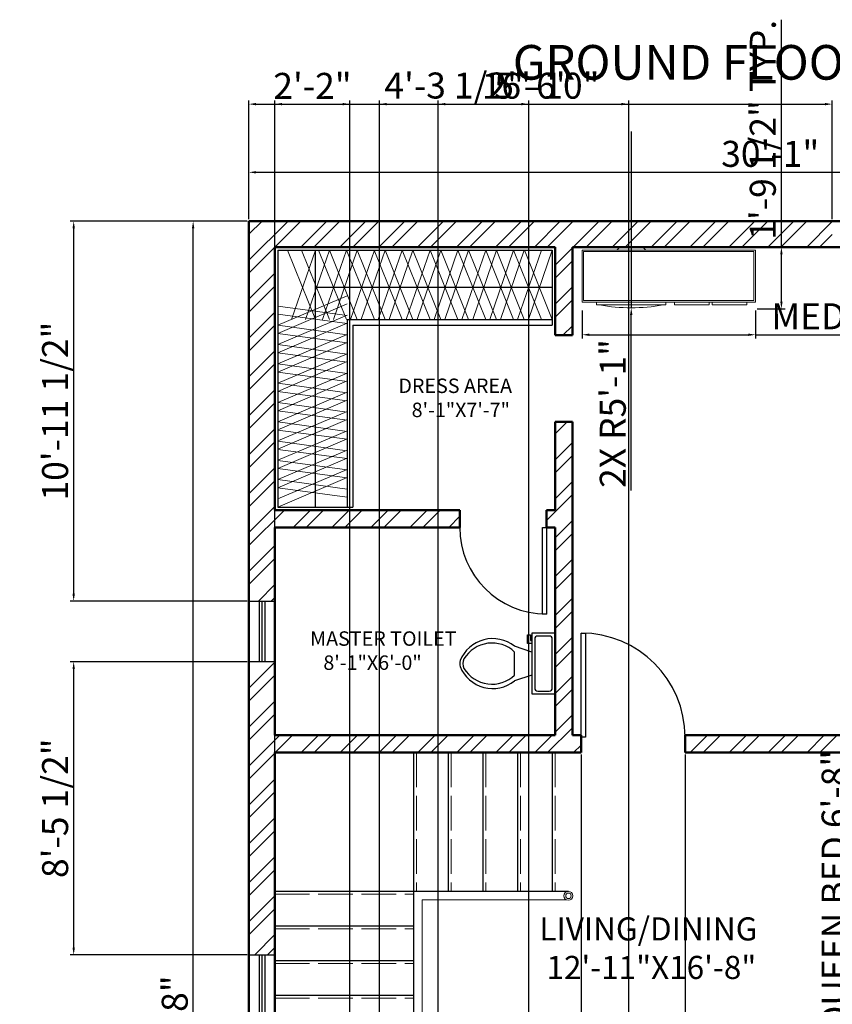
# Model space of a CAD drawing. Units: inches. Extents: x 635 to 1184, y 1837 to 2697.
# Tile 5 of 6: x 635 to 916, y 2356 to 2697. Entities that reach past the tile are written whole.
import ezdxf

# ---------------------------------------------------------------- set-up
doc = ezdxf.new("R2010")
doc.units = ezdxf.units.IN
doc.linetypes.add('ACAD_ISO02W100', pattern=[15, 12, -3])
for name, color, linetype, lineweight in [('A-ANNO-DIMS', 2, 'Continuous', 18), ('A-ANNO-TEXT', 7, 'Continuous', 25), ('A-AREA-IDEN', 7, 'Continuous', 25), ('A-CSWK', 8, 'Continuous', 25), ('A-CSWK-PATT', 252, 'Continuous', 13), ('A-DOOR', 4, 'Continuous', 25), ('A-FLOR-FIXT', 8, 'Continuous', 25), ('A-FLOR-RAIL', 7, 'Continuous', 18), ('A-FLOR-STRS', 7, 'Continuous', 25), ('A-FLOR-STRS-HIDN', 8, 'ACAD_ISO02W100', 13), ('A-FURN', 8, 'Continuous', 18), ('A-GLAZ', 244, 'Continuous', 25), ('A-WALL', 7, 'Continuous', 50), ('A-WALL-PATT', 252, 'Continuous', 13)]:
    doc.layers.add(name, color=color, linetype=linetype, lineweight=lineweight)
doc.styles.get("Standard").update_dxf_attribs({"font": 'arial.ttf'})
doc.dimstyles.new('ISO-25', dxfattribs={"dimtxt": 9, "dimasz": 2.5, "dimexe": 1.25, "dimexo": 0.625, "dimtad": 1, "dimlunit": 3, "dimtxsty": 'Standard', "dimcen": 2.5, "dimadec": 0, "dimazin": 0, "dimtfac": 1, "dimtmove": 0, "dimatfit": 3, "dimfxl": 1, "dimarcsym": 0})

# ---------------------------------------------------------------- blocks, each defined once
blk = doc.blocks.new('*U3')
for p, q in [((0, 0), (0, -6)), ((40, 0), (40, -6))]:
    blk.add_line(p, q)
blk.add_lwpolyline([(0, 0), (0, 40), (1.75, 40), (1.75, 0)], close=True)
blk.add_arc((0, 0), 40, 0, 90)
blk = doc.blocks.new('*U5')
for p, q in [((-40, 0), (-40, 6)), ((0, 0), (0, 6))]:
    blk.add_line(p, q)
blk.add_lwpolyline([(0, 0), (0, -40), (-1.75, -40), (-1.75, 0)], close=True)
blk.add_arc((0, 0), 40, 180, 270)
blk = doc.blocks.new('*U8')
for p, q in [((9.5, -6), (9.5, -2)), ((-10, -8.5), (-8, -8.5)), ((-10, -9.5), (-10, -8.5)), ((-7, -9.5), (-10, -9.5)), ((-8, -8.5), (-8, -8)), ((-7, -8), (-7, -9.5)), ((-4, -8), (-6, -14)), ((4, -8), (6, -14)), ((4, -14), (-4, -14))]:
    blk.add_line(p, q)
blk.add_lwpolyline([(10.5, -8), (10.5, 0), (-10.5, 0), (-10.5, -8)], close=True)
for points in [[(-9.5, -2), (-9.5, -6)], [(8.5, -1), (-8.5, -1)], [(-8.5, -7), (8.5, -7)]]:
    blk.add_lwpolyline(points)
for centre, radius, start, end in [((-8.62, -1.88), 0.884, 81.8699, 188.1301), ((8.62, -1.88), 0.884, 351.8699, 98.1301), ((-8.62, -6.12), 0.884, 171.8699, 278.1301), ((8.62, -6.12), 0.884, 261.8699, 8.1301), ((3.52, -21.58), 12.17, 141.4691, 247.9714), ((4.2, -21.82), 11.33, 136.3677, 238.9468), ((-3.52, -21.58), 12.17, 292.0284, 38.5307), ((-4.2, -21.82), 11.33, 301.053, 43.6321), ((0, -27.88), 4, 245.7318, 294.2682), ((0, -29), 4, 254.8605, 285.1395)]:
    blk.add_arc(centre, radius, start, end)
blk = doc.blocks.new('Entertainment Center')
for p, q in [((-4, 0), (-5, -1)), ((4, 0), (-4, 0)), ((5, -1), (4, 0)), ((-17, -19), (-17, -1)), ((-17, -1), (43, -1)), ((-16.5, -18.5), (-16.5, -1.5)), ((-16.5, -1.5), (42.5, -1.5)), ((42.5, -1.5), (42.5, -18.5)), ((43, -1), (43, -19)), ((43, -19), (-17, -19)), ((42.5, -18.5), (-16.5, -18.5)), ((-12, -20), (-12, -19)), ((12, -20), (-12, -20)), ((12, -19), (12, -20)), ((15, -20), (15, -19)), ((27, -20), (15, -20)), ((27, -19), (27, -20)), ((28, -20), (28, -19)), ((40, -20), (28, -20)), ((40, -19), (40, -20))]:
    blk.add_line(p, q)
blk.add_arc((0, 40), 61, 259.6111, 280.3889)
blk = doc.blocks.new('*D17')
at = {"layer": 'A-ANNO-DIMS', "color": 0, "lineweight": -2, "transparency": 16777216}
for p, q in [((713.66, 2627.14), (693.72, 2627.14)), ((694.97, 2056.46), (694.97, 2624.64)), ((713.66, 2053.96), (693.72, 2053.96))]:
    blk.add_line(p, q, dxfattribs=at)
at = {"layer": 'A-ANNO-DIMS', "color": 0, "transparency": 16777216}
for points in [[(694.56, 2624.64), (695.39, 2624.64), (694.97, 2627.14)], [(694.56, 2056.46), (695.39, 2056.46), (694.97, 2053.96)]]:
    blk.add_solid(points, dxfattribs=at)
at = {"layer": 'DEFPOINTS', "color": 0, "transparency": 16777216}
for p in [(694.97, 2627.14), (714.28, 2627.14), (714.28, 2053.96)]:
    blk.add_point(p, dxfattribs=at)
at = {"layer": 'A-ANNO-DIMS', "color": 0, "transparency": 16777216, "insert": (689.75, 2340.55), "char_height": 9, "attachment_point": 5, "rotation": 90}
blk.add_mtext('47\'-9.18"', dxfattribs=at)
blk = doc.blocks.new('*D18')
at = {"layer": 'A-ANNO-DIMS', "color": 0, "lineweight": -2, "transparency": 16777216}
for p, q in [((714.28, 2627.77), (714.28, 2645.3)), ((1075.28, 2627.77), (1075.28, 2645.3)), ((716.78, 2644.05), (1072.78, 2644.05))]:
    blk.add_line(p, q, dxfattribs=at)
at = {"layer": 'A-ANNO-DIMS', "color": 0, "transparency": 16777216}
for points in [[(716.78, 2644.46), (716.78, 2643.63), (714.28, 2644.05)], [(1072.78, 2644.46), (1072.78, 2643.63), (1075.28, 2644.05)]]:
    blk.add_solid(points, dxfattribs=at)
at = {"layer": 'DEFPOINTS', "color": 0, "transparency": 16777216}
for p in [(1075.28, 2644.05), (714.28, 2627.14), (1075.28, 2627.14)]:
    blk.add_point(p, dxfattribs=at)
at = {"layer": 'A-ANNO-DIMS', "color": 0, "transparency": 16777216, "insert": (894.78, 2649.27), "char_height": 9, "attachment_point": 5}
blk.add_mtext('30\'-1"', dxfattribs=at)
blk = doc.blocks.new('WIN-21IN')
for p, q in [((3.5, 21), (3.5, 0)), ((4.5, 21), (4.5, 0)), ((5.5, 21), (5.5, 0))]:
    blk.add_line(p, q)
blk.add_lwpolyline([(0, 21), (9, 21), (9, 0), (0, 0)], close=True)
blk = doc.blocks.new('WIN-60IN')
for p, q in [((0, 5.5), (60, 5.5)), ((0, 4.5), (60, 4.5)), ((0, 3.5), (60, 3.5))]:
    blk.add_line(p, q)
blk.add_lwpolyline([(0, 9), (60, 9), (60, 0), (0, 0)], close=True)
blk = doc.blocks.new('*D29')
at = {"layer": 'A-ANNO-DIMS', "color": 0, "lineweight": -2, "transparency": 16777216}
for p, q in [((829.66, 2596.18), (829.66, 2586.56)), ((889.66, 2596.18), (889.66, 2586.56)), ((832.16, 2587.81), (887.16, 2587.81)), ((889.66, 2587.81), (1024, 2587.81))]:
    blk.add_line(p, q, dxfattribs=at)
at = {"layer": 'A-ANNO-DIMS', "color": 0, "transparency": 16777216}
for points in [[(832.16, 2588.23), (832.16, 2587.39), (829.66, 2587.81)], [(887.16, 2588.23), (887.16, 2587.39), (889.66, 2587.81)]]:
    blk.add_solid(points, dxfattribs=at)
at = {"layer": 'DEFPOINTS', "color": 0, "transparency": 16777216}
for p in [(829.66, 2596.81), (889.66, 2596.81), (889.66, 2587.81)]:
    blk.add_point(p, dxfattribs=at)
at = {"layer": 'A-ANNO-DIMS', "color": 0, "transparency": 16777216, "insert": (958.08, 2593.03), "char_height": 9, "attachment_point": 5}
blk.add_mtext('MEDIA UNIT 5\'-0" TYP.', dxfattribs=at)
blk = doc.blocks.new('*D30')
at = {"layer": 'A-ANNO-DIMS', "color": 0, "lineweight": -2, "transparency": 16777216}
for p, q in [((898.66, 2618.14), (898.66, 2696.88)), ((890.29, 2618.14), (899.91, 2618.14)), ((898.66, 2599.31), (898.66, 2615.64)), ((890.29, 2596.81), (899.91, 2596.81))]:
    blk.add_line(p, q, dxfattribs=at)
at = {"layer": 'A-ANNO-DIMS', "color": 0, "transparency": 16777216}
for points in [[(898.25, 2615.64), (899.08, 2615.64), (898.66, 2618.14)], [(898.25, 2599.31), (899.08, 2599.31), (898.66, 2596.81)]]:
    blk.add_solid(points, dxfattribs=at)
at = {"layer": 'DEFPOINTS', "color": 0, "transparency": 16777216}
for p in [(889.66, 2618.14), (898.66, 2618.14), (889.66, 2596.81)]:
    blk.add_point(p, dxfattribs=at)
at = {"layer": 'A-ANNO-DIMS', "color": 0, "transparency": 16777216, "insert": (893.38, 2658.76), "char_height": 9, "attachment_point": 5, "rotation": 90}
blk.add_mtext('1\'-9 1/2" TYP.', dxfattribs=at)
blk = doc.blocks.new('*D35')
at = {"layer": 'A-ANNO-DIMS', "color": 0, "lineweight": -2, "transparency": 16777216}
for p, q in [((935.16, 2529.14), (922.53, 2529.14)), ((923.78, 2526.64), (923.78, 2451.64)), ((935.16, 2449.14), (922.53, 2449.14)), ((923.78, 2449.14), (923.78, 2343.94))]:
    blk.add_line(p, q, dxfattribs=at)
at = {"layer": 'A-ANNO-DIMS', "color": 0, "transparency": 16777216}
for points in [[(923.37, 2526.64), (924.2, 2526.64), (923.78, 2529.14)], [(923.37, 2451.64), (924.2, 2451.64), (923.78, 2449.14)]]:
    blk.add_solid(points, dxfattribs=at)
at = {"layer": 'DEFPOINTS', "color": 0, "transparency": 16777216}
for p in [(935.78, 2529.14), (923.78, 2449.14), (935.78, 2449.14)]:
    blk.add_point(p, dxfattribs=at)
at = {"layer": 'A-ANNO-DIMS', "color": 0, "transparency": 16777216, "insert": (918.23, 2395.29), "char_height": 9, "attachment_point": 5, "rotation": 90}
blk.add_mtext('QUEEN BED 6\'-8"', dxfattribs=at)
blk = doc.blocks.new('*D42')
at = {"layer": 'A-ANNO-DIMS', "color": 0, "lineweight": -2, "transparency": 16777216}
for p, q in [((713.66, 2474.64), (652.36, 2474.64)), ((653.61, 2375.64), (653.61, 2472.14)), ((713.66, 2373.14), (652.36, 2373.14))]:
    blk.add_line(p, q, dxfattribs=at)
at = {"layer": 'A-ANNO-DIMS', "color": 0, "transparency": 16777216}
for points in [[(653.2, 2472.14), (654.03, 2472.14), (653.61, 2474.64)], [(653.2, 2375.64), (654.03, 2375.64), (653.61, 2373.14)]]:
    blk.add_solid(points, dxfattribs=at)
at = {"layer": 'DEFPOINTS', "color": 0, "transparency": 16777216}
for p in [(653.61, 2474.64), (714.28, 2474.64), (714.28, 2373.14)]:
    blk.add_point(p, dxfattribs=at)
at = {"layer": 'A-ANNO-DIMS', "color": 0, "transparency": 16777216, "insert": (648.34, 2423.89), "char_height": 9, "attachment_point": 5, "rotation": 90}
blk.add_mtext('8\'-5 1/2"', dxfattribs=at)
blk = doc.blocks.new('*D43')
at = {"layer": 'A-ANNO-DIMS', "color": 0, "lineweight": -2, "transparency": 16777216}
for p, q in [((713.66, 2627.14), (652.36, 2627.14)), ((653.61, 2498.14), (653.61, 2624.64)), ((713.66, 2495.64), (652.36, 2495.64))]:
    blk.add_line(p, q, dxfattribs=at)
at = {"layer": 'A-ANNO-DIMS', "color": 0, "transparency": 16777216}
for points in [[(653.2, 2624.64), (654.03, 2624.64), (653.61, 2627.14)], [(653.2, 2498.14), (654.03, 2498.14), (653.61, 2495.64)]]:
    blk.add_solid(points, dxfattribs=at)
at = {"layer": 'DEFPOINTS', "color": 0, "transparency": 16777216}
for p in [(653.61, 2627.14), (714.28, 2627.14), (714.28, 2495.64)]:
    blk.add_point(p, dxfattribs=at)
at = {"layer": 'A-ANNO-DIMS', "color": 0, "transparency": 16777216, "insert": (648.34, 2561.39), "char_height": 9, "attachment_point": 5, "rotation": 90}
blk.add_mtext('10\'-11 1/2"', dxfattribs=at)
blk = doc.blocks.new('*D44')
at = {"layer": 'A-ANNO-DIMS', "color": 0, "lineweight": -2, "transparency": 16777216}
for p, q in [((714.28, 2627.77), (714.28, 2668.89)), ((916.28, 2627.77), (916.28, 2668.89)), ((716.78, 2667.64), (913.78, 2667.64))]:
    blk.add_line(p, q, dxfattribs=at)
at = {"layer": 'A-ANNO-DIMS', "color": 0, "transparency": 16777216}
for points in [[(716.78, 2668.06), (716.78, 2667.23), (714.28, 2667.64)], [(913.78, 2668.06), (913.78, 2667.23), (916.28, 2667.64)]]:
    blk.add_solid(points, dxfattribs=at)
at = {"layer": 'DEFPOINTS', "color": 0, "transparency": 16777216}
for p in [(916.28, 2667.64), (714.28, 2627.14), (916.28, 2627.14)]:
    blk.add_point(p, dxfattribs=at)
at = {"layer": 'A-ANNO-DIMS', "color": 0, "transparency": 16777216, "insert": (815.28, 2672.86), "char_height": 9, "attachment_point": 5}
blk.add_mtext('16\'-10"', dxfattribs=at)
blk = doc.blocks.new('*D56')
at = {"layer": 'A-ANNO-DIMS', "color": 0, "lineweight": -2, "transparency": 16777216}
for p, q in [((759.51, 2116.34), (759.51, 2668.89)), ((811.15, 2116.34), (811.15, 2668.89)), ((762.01, 2667.64), (808.65, 2667.64))]:
    blk.add_line(p, q, dxfattribs=at)
at = {"layer": 'A-ANNO-DIMS', "color": 0, "transparency": 16777216}
for points in [[(762.01, 2668.06), (762.01, 2667.23), (759.51, 2667.64)], [(808.65, 2668.06), (808.65, 2667.23), (811.15, 2667.64)]]:
    blk.add_solid(points, dxfattribs=at)
at = {"layer": 'DEFPOINTS', "color": 0, "transparency": 16777216}
for p in [(811.15, 2667.64), (759.51, 2115.72), (811.15, 2115.72)]:
    blk.add_point(p, dxfattribs=at)
at = {"layer": 'A-ANNO-DIMS', "color": 0, "transparency": 16777216, "insert": (785.33, 2672.92), "char_height": 9, "attachment_point": 5}
blk.add_mtext('4\'-3 1/2"', dxfattribs=at)
blk = doc.blocks.new('*D59')
at = {"layer": 'A-ANNO-DIMS', "color": 0, "lineweight": -2, "transparency": 16777216}
for p, q in [((723.28, 2181.16), (723.28, 2668.89)), ((749.28, 2181.16), (749.28, 2668.89)), ((725.78, 2667.64), (746.78, 2667.64))]:
    blk.add_line(p, q, dxfattribs=at)
at = {"layer": 'A-ANNO-DIMS', "color": 0, "transparency": 16777216}
for points in [[(725.78, 2668.06), (725.78, 2667.23), (723.28, 2667.64)], [(746.78, 2668.06), (746.78, 2667.23), (749.28, 2667.64)]]:
    blk.add_solid(points, dxfattribs=at)
at = {"layer": 'DEFPOINTS', "color": 0, "transparency": 16777216}
for p in [(749.28, 2667.64), (723.28, 2180.53), (749.28, 2180.53)]:
    blk.add_point(p, dxfattribs=at)
at = {"layer": 'A-ANNO-DIMS', "color": 0, "transparency": 16777216, "insert": (736.28, 2672.79), "char_height": 9, "attachment_point": 5}
blk.add_mtext('2\'-2"', dxfattribs=at)
blk = doc.blocks.new('*D60')
at = {"layer": 'A-ANNO-DIMS', "color": 0, "lineweight": -2, "transparency": 16777216}
for p, q in [((779.78, 2243.77), (779.78, 2668.89)), ((845.78, 2243.77), (845.78, 2668.89)), ((782.28, 2667.64), (843.28, 2667.64))]:
    blk.add_line(p, q, dxfattribs=at)
at = {"layer": 'A-ANNO-DIMS', "color": 0, "transparency": 16777216}
for points in [[(782.28, 2668.06), (782.28, 2667.23), (779.78, 2667.64)], [(843.28, 2668.06), (843.28, 2667.23), (845.78, 2667.64)]]:
    blk.add_solid(points, dxfattribs=at)
at = {"layer": 'DEFPOINTS', "color": 0, "transparency": 16777216}
for p in [(845.78, 2667.64), (779.78, 2243.14), (845.78, 2243.14)]:
    blk.add_point(p, dxfattribs=at)
at = {"layer": 'A-ANNO-DIMS', "color": 0, "transparency": 16777216, "insert": (812.78, 2672.86), "char_height": 9, "attachment_point": 5}
blk.add_mtext('5\'-6"', dxfattribs=at)
blk = doc.blocks.new('*D62')
at = {"layer": 'A-ANNO-DIMS', "color": 0, "lineweight": -2, "transparency": 16777216}
for p, q in [((829.28, 2442.52), (829.28, 1843.99)), ((865.28, 2442.52), (865.28, 1843.99)), ((831.78, 1845.24), (862.78, 1845.24))]:
    blk.add_line(p, q, dxfattribs=at)
at = {"layer": 'A-ANNO-DIMS', "color": 0, "transparency": 16777216}
for points in [[(831.78, 1845.65), (831.78, 1844.82), (829.28, 1845.24)], [(862.78, 1845.65), (862.78, 1844.82), (865.28, 1845.24)]]:
    blk.add_solid(points, dxfattribs=at)
at = {"layer": 'DEFPOINTS', "color": 0, "transparency": 16777216}
for p in [(829.28, 2443.14), (865.28, 2443.14), (865.28, 1845.24)]:
    blk.add_point(p, dxfattribs=at)
at = {"layer": 'A-ANNO-DIMS', "color": 0, "transparency": 16777216, "insert": (847.28, 1850.46), "char_height": 9, "attachment_point": 5}
blk.add_mtext('3\'-0"', dxfattribs=at)
blk = doc.blocks.new('*D66')
at = {"layer": 'A-ANNO-DIMS', "color": 0, "lineweight": -2, "transparency": 16777216}
for p, q in [((846.66, 2658.14), (846.66, 2597.14)), ((846.66, 2533.9), (846.66, 2594.64))]:
    blk.add_line(p, q, dxfattribs=at)
at = {"layer": 'A-ANNO-DIMS', "color": 0, "transparency": 16777216}
blk.add_solid([(846.24, 2594.64), (847.08, 2594.64), (846.66, 2597.14)], dxfattribs=at)
at = {"layer": 'DEFPOINTS', "color": 0, "transparency": 16777216}
for p in [(846.66, 2658.14), (846.66, 2597.14)]:
    blk.add_point(p, dxfattribs=at)
at = {"layer": 'A-ANNO-DIMS', "color": 0, "transparency": 16777216, "insert": (841.44, 2560.54), "char_height": 9, "attachment_point": 5, "rotation": 89.9972}
blk.add_mtext('2X R5\'-1"', dxfattribs=at)

msp = doc.modelspace()

# ---------------------------------------------------------------- hatches: boundary and pattern name
at = {"layer": 'A-CSWK-PATT'}
h = msp.add_hatch(dxfattribs=at)
h.set_pattern_fill('ANSI31', color=256, scale=2.81766, angle=66.8789, style=0)
h.paths.add_polyline_path([(819.632, 2593.142), (809.992, 2617.142), (732.168, 2617.142), (741.809, 2593.142)])
h = msp.add_hatch(dxfattribs=at)
h.set_pattern_fill('ANSI31', color=256, scale=2.87254, angle=26.0933, style=0)
h.paths.add_polyline_path([(819.632, 2617.142), (811.38, 2593.142), (733.557, 2593.142), (741.809, 2617.142)])
h = msp.add_hatch(dxfattribs=at)
h.set_pattern_fill('ANSI31', color=256, scale=2.81627, angle=66.9495, style=0)
h.paths.add_polyline_path([(815.902, 2593.142), (806.261, 2617.142), (738.078, 2617.142), (747.719, 2593.142)])
h = msp.add_hatch(dxfattribs=at)
h.set_pattern_fill('ANSI31', color=256, scale=2.87054, angle=25.977, style=0)
h.paths.add_polyline_path([(815.902, 2617.142), (807.65, 2593.142), (739.467, 2593.142), (747.719, 2617.142)])
h = msp.add_hatch(dxfattribs=at)
h.set_pattern_fill('ANSI31', color=256, scale=1.93691, angle=-22.0365, style=0)
h.paths.add_polyline_path([(724.282, 2530.604), (748.282, 2540.859), (748.282, 2601.67), (724.282, 2591.415)])
h = msp.add_hatch(dxfattribs=at)
h.set_pattern_fill('ANSI31', color=256, scale=1.933247, angle=-21.78187, style=0)
h.paths.add_polyline_path([(724.282, 2527.792), (748.282, 2538.047), (748.282, 2598.858), (724.282, 2588.603)])
h = msp.add_hatch(dxfattribs=at)
h.set_pattern_fill('ANSI31', color=256, scale=2.083634, angle=127.0962, style=0)
h.paths.add_polyline_path([(748.282, 2594.792), (724.282, 2598.094), (724.282, 2537.283), (748.282, 2533.981)])
h = msp.add_hatch(dxfattribs=at)
h.set_pattern_fill('ANSI31', color=256, scale=2.085098, angle=127.3917, style=0)
h.paths.add_polyline_path([(748.282, 2591.98), (724.282, 2595.282), (724.282, 2534.471), (748.282, 2531.17)])
at = {"layer": 'A-WALL-PATT'}
h = msp.add_hatch(dxfattribs=at)
h.set_pattern_fill('ANSI32', color=256)
h.paths.add_polyline_path([(723.282, 2313.142), (714.282, 2313.142), (714.282, 2234.142), (718.782, 2234.142), (723.282, 2234.142), (723.282, 2237.142), (779.782, 2237.142), (779.782, 2243.142), (723.282, 2243.142)])
h.paths.add_polyline_path([(926.282, 2320.142), (920.282, 2320.142), (920.282, 2243.142), (845.782, 2243.142), (845.782, 2237.142), (920.282, 2237.142), (920.282, 2093.142), (860.282, 2093.142), (860.282, 2165.142), (854.282, 2165.142), (854.282, 2093.142), (818.782, 2093.142), (818.782, 2084.142), (929.282, 2084.142), (929.282, 2156.142), (932.282, 2156.142), (932.282, 2165.142), (926.282, 2165.142)])
h.paths.add_polyline_path([(1075.282, 2250.443), (1066.282, 2250.443), (1066.282, 2233.442), (1075.282, 2233.442)])
h.paths.add_polyline_path([(1075.282, 2173.442), (1066.282, 2173.442), (1066.282, 2165.142), (1057.782, 2165.142), (1057.782, 2156.142), (1075.282, 2156.142)])
h.paths.add_polyline_path([(997.782, 2165.142), (980.282, 2165.142), (980.282, 2156.142), (997.782, 2156.142)])
h.paths.add_polyline_path([(1075.282, 2338.142), (1066.282, 2338.142), (1066.282, 2310.443), (1075.282, 2310.443)])
h.paths.add_polyline_path([(758.782, 2093.142), (723.282, 2093.142), (723.282, 2154.642), (714.282, 2154.642), (714.282, 2084.142), (758.782, 2084.142)])
h.paths.add_polyline_path([(723.282, 2204.142), (714.282, 2204.142), (714.282, 2175.642), (723.282, 2175.642)])
h.paths.add_polyline_path([(1075.282, 2404.069), (1066.282, 2404.069), (1066.282, 2383.142), (970.282, 2383.142), (970.282, 2386.142), (964.282, 2386.142), (964.282, 2383.142), (926.282, 2383.142), (926.282, 2389.142), (920.282, 2389.142), (920.282, 2368.142), (926.282, 2368.142), (926.282, 2377.142), (1066.282, 2377.142), (1066.282, 2374.142), (1075.282, 2374.142)])
h.paths.add_polyline_path([(926.282, 2443.142), (964.282, 2443.142), (964.282, 2416.142), (970.282, 2416.142), (970.282, 2443.142), (1066.282, 2443.142), (1066.282, 2425.069), (1075.282, 2425.069), (1075.282, 2503.642), (1066.282, 2503.642), (1066.282, 2449.142), (865.282, 2449.142), (865.282, 2443.142), (920.282, 2443.142), (920.282, 2416.142), (926.282, 2416.142)])
h.paths.add_polyline_path([(829.282, 2449.142), (826.282, 2449.142), (826.282, 2527.142), (826.282, 2557.642), (820.282, 2557.642), (820.282, 2527.142), (817.282, 2527.142), (817.282, 2521.142), (820.282, 2521.142), (820.282, 2449.142), (723.282, 2449.142), (723.282, 2474.642), (714.282, 2474.642), (714.282, 2373.142), (723.282, 2373.142), (723.282, 2443.142), (829.282, 2443.142)])
h.paths.add_polyline_path([(787.282, 2527.142), (723.282, 2527.142), (723.282, 2618.142), (820.282, 2618.142), (820.282, 2587.642), (826.282, 2587.642), (826.282, 2618.142), (916.282, 2618.142), (916.282, 2627.142), (714.282, 2627.142), (714.282, 2495.642), (723.282, 2495.642), (723.282, 2521.142), (787.282, 2521.142)])
h.paths.add_polyline_path([(1075.282, 2627.142), (976.282, 2627.142), (976.282, 2618.142), (1066.282, 2618.142), (1066.282, 2563.642), (1075.282, 2563.642)])

# ---------------------------------------------------------------- linework, layer by layer
at = {"layer": 'A-CSWK'}
for p, q in [((724.282, 2617.142), (819.282, 2617.142)), ((724.282, 2617.142), (724.282, 2528.142)), ((737.282, 2528.142), (737.282, 2617.142)), ((819.282, 2617.142), (819.282, 2591.142)), ((819.282, 2604.142), (737.282, 2604.142)), ((748.282, 2593.142), (748.282, 2528.142)), ((748.282, 2593.142), (819.282, 2593.142)), ((750.282, 2591.142), (819.282, 2591.142)), ((750.282, 2591.142), (750.282, 2528.142)), ((724.282, 2528.142), (750.282, 2528.142))]:
    msp.add_line(p, q, dxfattribs=at)
at = {"layer": 'A-CSWK-PATT'}
for p, q in [((737.282, 2593.142), (727.642, 2617.142)), ((737.282, 2617.142), (729.03, 2593.142))]:
    msp.add_line(p, q, dxfattribs=at)
at = {"layer": 'A-FLOR-RAIL'}
for q in [(774.282, 2292.647), (824.324, 2392.142)]:
    msp.add_line((774.282, 2392.142), q, dxfattribs=at)
for radius in [1.559, 0.959]:
    msp.add_circle((824.919, 2393.583), radius, dxfattribs=at)
at = {"layer": 'A-FLOR-STRS'}
for p, q in [((771.282, 2443.142), (771.282, 2292.661)), ((783.282, 2443.142), (783.282, 2395.142)), ((795.282, 2443.142), (795.282, 2395.142)), ((807.282, 2443.142), (807.282, 2395.142)), ((819.282, 2443.142), (819.282, 2395.142)), ((723.282, 2395.142), (824.919, 2395.142)), ((723.282, 2383.142), (771.282, 2383.142)), ((723.282, 2371.142), (771.282, 2371.142)), ((723.282, 2359.142), (771.282, 2359.142))]:
    msp.add_line(p, q, dxfattribs=at)
at = {"layer": 'A-FLOR-STRS-HIDN'}
for p, q in [((772.282, 2443.142), (772.282, 2395.142)), ((784.282, 2443.142), (784.282, 2395.142)), ((796.282, 2443.142), (796.282, 2395.142)), ((808.282, 2443.142), (808.282, 2395.142)), ((820.282, 2443.142), (820.282, 2395.142)), ((723.282, 2394.142), (771.282, 2394.142)), ((723.282, 2382.142), (771.282, 2382.142)), ((723.282, 2370.142), (771.282, 2370.142)), ((723.282, 2358.142), (771.282, 2358.142))]:
    msp.add_line(p, q, dxfattribs=at)
at = {"layer": 'A-WALL'}
for p, q in [((714.282, 2627.142), (714.282, 2234.142)), ((714.282, 2627.142), (1075.282, 2627.142)), ((723.282, 2618.142), (820.282, 2618.142)), ((723.282, 2618.142), (723.282, 2527.142)), ((820.282, 2618.142), (820.282, 2587.642)), ((826.282, 2618.142), (826.282, 2587.642)), ((826.282, 2618.142), (1066.282, 2618.142)), ((826.282, 2587.642), (820.282, 2587.642)), ((826.282, 2557.642), (820.282, 2557.642)), ((820.282, 2557.642), (820.282, 2527.142)), ((826.282, 2557.642), (826.282, 2527.142)), ((723.282, 2527.142), (787.282, 2527.142)), ((787.282, 2527.142), (787.282, 2521.142)), ((817.282, 2527.142), (817.282, 2521.142)), ((817.282, 2527.142), (820.282, 2527.142)), ((826.282, 2527.142), (826.282, 2449.142)), ((723.282, 2521.142), (787.282, 2521.142)), ((723.282, 2521.142), (723.282, 2449.142)), ((817.282, 2521.142), (820.282, 2521.142)), ((820.282, 2521.142), (820.282, 2449.142)), ((723.282, 2449.142), (820.282, 2449.142)), ((826.282, 2449.142), (829.282, 2449.142)), ((829.282, 2449.142), (829.282, 2443.142)), ((865.282, 2449.142), (865.282, 2443.142)), ((865.282, 2449.142), (1066.282, 2449.142)), ((723.282, 2443.142), (829.282, 2443.142)), ((723.282, 2443.142), (723.282, 2243.142)), ((865.282, 2443.142), (920.282, 2443.142))]:
    msp.add_line(p, q, dxfattribs=at)

# ---------------------------------------------------------------- block references
at = {"layer": 'A-DOOR'}
for name, p, xscale, yscale, zscale in [('*U5', (817.282, 2521.142), 0.7499999999999997, 0.7499999999999997, 0.7499999999999997), ('*U3', (829.282, 2448.542), 0.8999999999999996, 0.8999999999999996, 0.8999999999999996)]:
    msp.add_blockref(name, p, dxfattribs=dict(at, xscale=xscale, yscale=yscale, zscale=zscale))
at = {"layer": 'A-FLOR-FIXT', "rotation": 270}
msp.add_blockref('*U8', (820.282, 2473.97), dxfattribs=at)
at = {"layer": 'A-FURN'}
msp.add_blockref('Entertainment Center', (846.663, 2618.142), dxfattribs=at)
at = {"layer": 'A-GLAZ'}
msp.add_blockref('WIN-21IN', (714.282, 2474.642), dxfattribs=at)
at = {"layer": 'A-GLAZ', "rotation": 270.0000000000011}
msp.add_blockref('WIN-60IN', (714.282, 2373.142), dxfattribs=at)

# ---------------------------------------------------------------- texts
at = {"layer": 'A-ANNO-TEXT', "insert": (805.654, 2688.104), "char_height": 12, "attachment_point": 1}
msp.add_mtext_dynamic_manual_height_columns('GROUND FLOOR PLAN ', width=188.74888, gutter_width=12.5, heights=[0], dxfattribs=at)
at = {"layer": 'A-AREA-IDEN', "attachment_point": 1}
for s, width, insert, char_height in [('DRESS AREA\\P   8\'-1"X7\'-7"', 45.78341, (766.043, 2572.642), 5), ('MASTER TOILET\\P   8\'-1"X6\'-0"', 55.22623, (735.479, 2485.142), 5), ('LIVING/DINING\\P 12\'-11"X16\'-8"', 78.58477, (814.867, 2386.13), 8)]:
    msp.add_mtext_dynamic_manual_height_columns(s, width=width, gutter_width=12.5, heights=[0], dxfattribs=dict(at, insert=insert, char_height=char_height))

# ---------------------------------------------------------------- dimensions: what is measured, and where the dimension line sits
at = {"layer": 'A-ANNO-DIMS'}
for base, p1, p2, angle, text, picture, middle in [((898.663, 2618.142), (889.663, 2596.809), (889.663, 2618.142), 90, '<> TYP.', '*D30', (893.384, 2658.759)), ((923.782, 2449.142), (935.782, 2529.142), (935.782, 2449.142), 270, 'QUEEN BED <>', '*D35', (918.227, 2395.289))]:
    dim = msp.add_linear_dim(base=base, p1=p1, p2=p2, angle=angle, text=text, dimstyle='ISO-25', override={"dimdec": 1, "dimlfac": 1, "dimrnd": 0, "dimzin": 1, "dimdsep": 46, "dimlunit": 4, "dimfrac": 2}, dxfattribs=at)
    dim.commit()
    dim.dimension.update_dxf_attribs({"geometry": picture, "text_midpoint": middle})
for base, p1, p2, override, picture, middle in [((811.15, 2667.642), (759.513, 2115.719), (811.15, 2115.719), {"dimdec": 1, "dimlfac": 1, "dimrnd": 0, "dimzin": 1, "dimdsep": 46, "dimlunit": 4, "dimfrac": 2}, '*D56', (785.331, 2672.923)), ((916.282, 2667.642), (714.282, 2627.142), (916.282, 2627.142), {"dimdec": 1, "dimlfac": 1, "dimrnd": 0, "dimzin": 1, "dimdsep": 46, "dimlunit": 4, "dimfrac": 2}, '*D44', (815.282, 2672.862)), ((749.282, 2667.642), (723.282, 2180.535), (749.282, 2180.535), {"dimdec": 1, "dimlfac": 1, "dimrnd": 0, "dimzin": 1, "dimdsep": 46, "dimlunit": 4, "dimfrac": 2}, '*D59', (736.282, 2672.785)), ((845.782, 2667.642), (779.782, 2243.142), (845.782, 2243.142), {"dimdec": 1, "dimlfac": 1, "dimrnd": 0, "dimzin": 1, "dimdsep": 46, "dimlunit": 4, "dimfrac": 2}, '*D60', (812.782, 2672.862)), ((1075.282, 2644.045), (714.282, 2627.142), (1075.282, 2627.142), {"dimclrd": 0, "dimclre": 0, "dimclrt": 0}, '*D18', (894.782, 2649.269)), ((865.282, 1845.237), (829.282, 2443.142), (865.282, 2443.142), {"dimdec": 1, "dimlfac": 1, "dimrnd": 0, "dimzin": 1, "dimdsep": 46, "dimlunit": 4, "dimfrac": 2}, '*D62', (847.282, 1850.461))]:
    dim = msp.add_linear_dim(base=base, p1=p1, p2=p2, dimstyle='ISO-25', override=override, dxfattribs=at)
    dim.commit()
    dim.dimension.update_dxf_attribs({"geometry": picture, "text_midpoint": middle})
dim = msp.add_radius_dim(center=(846.663, 2658.142), mpoint=(846.66, 2597.142), text='2X <>', dimstyle='ISO-25', override={"dimdec": 1, "dimlfac": 1, "dimrnd": 0, "dimzin": 1, "dimdsep": 46, "dimlunit": 4, "dimfrac": 2}, dxfattribs=at)
dim.commit()
dim.dimension.update_dxf_attribs({"geometry": '*D66', "text_midpoint": (846.658, 2560.542), "dimtype": 164})
for base, p1, p2, override, picture, middle in [((653.614, 2627.142), (714.282, 2495.642), (714.282, 2627.142), {"dimdec": 1, "dimlfac": 1, "dimrnd": 0, "dimzin": 1, "dimdsep": 46, "dimlunit": 4, "dimfrac": 2}, '*D43', (648.336, 2561.392)), ((694.972, 2627.142), (714.282, 2053.962), (714.282, 2627.142), {"dimclrd": 0, "dimclre": 0, "dimclrt": 0}, '*D17', (689.752, 2340.552)), ((653.614, 2474.642), (714.282, 2373.142), (714.282, 2474.642), {"dimdec": 1, "dimlfac": 1, "dimrnd": 0, "dimzin": 1, "dimdsep": 46, "dimlunit": 4, "dimfrac": 2}, '*D42', (648.336, 2423.892))]:
    dim = msp.add_linear_dim(base=base, p1=p1, p2=p2, angle=90, dimstyle='ISO-25', override=override, dxfattribs=at)
    dim.commit()
    dim.dimension.update_dxf_attribs({"geometry": picture, "text_midpoint": middle})
dim = msp.add_linear_dim(base=(889.663, 2587.809), p1=(829.663, 2596.809), p2=(889.663, 2596.809), text='MEDIA UNIT <> TYP.', dimstyle='ISO-25', override={"dimdec": 1, "dimlfac": 1, "dimrnd": 0, "dimzin": 1, "dimdsep": 46, "dimlunit": 4, "dimfrac": 2}, dxfattribs=at)
dim.commit()
dim.dimension.update_dxf_attribs({"geometry": '*D29', "text_midpoint": (958.081, 2593.029)})

doc.saveas('drawing.dxf')
